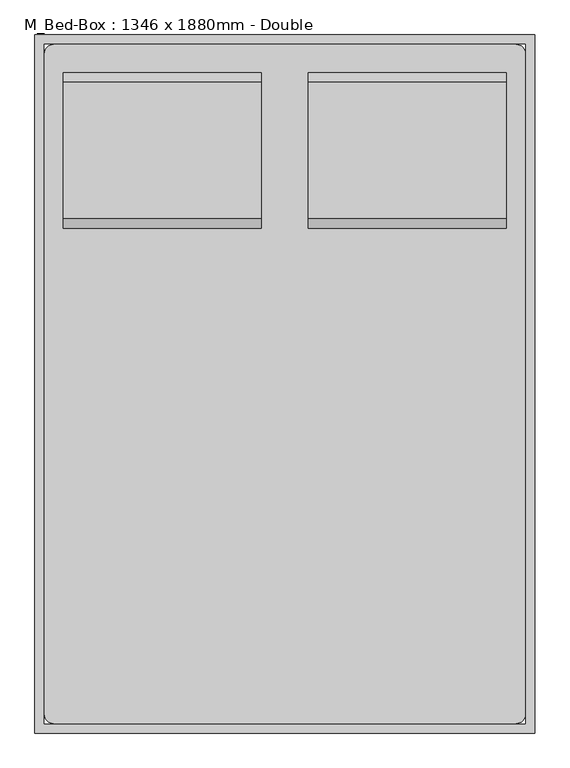
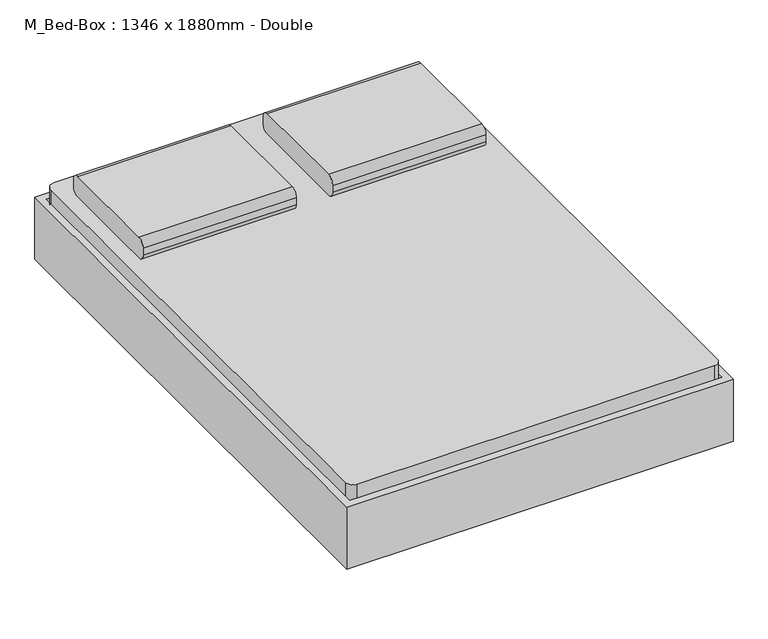
"""IFC4 building model written with IfcOpenShell, lengths in millimetres: furniture geometry, M_Bed-Box : 1346 x 1880mm - Double."""

from ifc_helpers import new_model, si_unit, point, frame, frame_2d, origin, place, context, project, spatial, polyline, circle_curve, trimmed, segment, composite_curve, outline, extrude, source, transform, mapped, element, save
from ifc_brep_helpers import plane_surface, cylinder_surface, revolved_surface, advanced_brep


def m_bed_box_1346_x_1880mm_double_52b0093e(model_context):
    return source(origin(), model_context, "Body", "SolidModel", [
        advanced_brep(
        [(-308.447541, -869.6295082, 196.85), (-308.447541, -869.6295082, 177.8), (-308.447541, -945.8295082, 177.8), (-308.447541, -945.8295082, 196.85), (-245.5113525, -869.6295082, 196.85), (-257.647541, -869.6295082, 177.8), (-257.647541, -945.8295082, 177.8), (-245.5113525, -945.8295082, 196.85), (-164.3115092, -869.6295082, 22.716374), (-181.5766725, -869.6295082, 14.6654962), (-181.5766725, -945.8295082, 14.6654962), (-164.3115092, -945.8295082, 22.716374), (-158.5564547, -869.6295082, 0.0), (-158.5564547, -869.6295082, 19.05), (-158.5564547, -945.8295082, 0.0), (-158.5564547, -945.8295082, 19.05), (-79.9439489, -869.6295082, 19.05), (-79.9439489, -869.6295082, 0.0), (-79.9439489, -945.8295082, 0.0), (-79.9439489, -945.8295082, 19.05), (-67.2439489, -869.6295082, 3.4029547), (-76.7689489, -869.6295082, 19.9007387), (-67.2439489, -945.8295082, 3.4029547), (-76.7689489, -945.8295082, 19.9007387), (-12.2513357, -869.6295082, 57.15), (-7.1469036, -869.6295082, 38.1), (-7.1469036, -945.8295082, 38.1), (-12.2513357, -945.8295082, 57.15), (690.5562537, -869.6295082, 57.15), (685.4518216, -869.6295082, 38.1), (685.4518216, -945.8295082, 38.1), (690.5562537, -945.8295082, 57.15), (755.0738669, -869.6295082, 19.9007387), (745.5488669, -869.6295082, 3.4029547), (745.5488669, -945.8295082, 3.4029547), (755.0738669, -945.8295082, 19.9007387), (758.2488669, -869.6295082, 0.0), (758.2488669, -869.6295082, 19.05), (758.2488669, -945.8295082, 0.0), (758.2488669, -945.8295082, 19.05), (836.8613728, -869.6295082, 19.05), (836.8613728, -869.6295082, 0.0), (836.8613728, -945.8295082, 0.0), (836.8613728, -945.8295082, 19.05), (859.8815906, -869.6295082, 14.6654962), (842.6164272, -869.6295082, 22.716374), (859.8815906, -945.8295082, 14.6654962), (842.6164272, -945.8295082, 22.716374), (923.8162705, -869.6295082, 196.85), (935.952459, -869.6295082, 177.8), (935.952459, -945.8295082, 177.8), (923.8162705, -945.8295082, 196.85), (986.752459, -869.6295082, 196.85), (986.752459, -945.8295082, 196.85), (986.752459, -945.8295082, 177.8), (986.752459, -869.6295082, 177.8)],
        [
            (0, 1),
            (1, 2),
            (2, 3),
            (3, 0),
            (0, 4),
            (4, 5),
            (5, 1),
            (5, 6),
            (6, 2),
            (6, 7),
            (7, 3),
            (7, 4),
            (4, 8),
            (8, 9),
            (9, 5),
            (9, 10),
            (10, 6),
            (10, 11),
            (11, 7),
            (11, 8),
            (12, 9, circle_curve(frame((-158.5564547, -869.6295082, 25.4), z_axis=(0.0, 1.0, 0.0), x_axis=(-0.9063077870366625, 0.0, -0.4226182617406725)), 25.4)),
            (8, 13, circle_curve(frame((-158.5564547, -869.6295082, 25.4), z_axis=(0.0, -1.0, 0.0), x_axis=(-0.9063077870366625, 0.0, -0.4226182617406725)), 6.35)),
            (13, 12),
            (14, 10, circle_curve(frame((-158.5564547, -945.8295082, 25.4), z_axis=(0.0, 1.0, 0.0), x_axis=(-0.9063077870366625, 0.0, -0.4226182617406725)), 25.4)),
            (12, 14),
            (15, 11, circle_curve(frame((-158.5564547, -945.8295082, 25.4), z_axis=(0.0, 1.0, 0.0), x_axis=(-0.9063077870366625, 0.0, -0.4226182617406725)), 6.35)),
            (14, 15),
            (15, 13),
            (13, 16),
            (16, 17),
            (17, 12),
            (17, 18),
            (18, 14),
            (18, 19),
            (19, 15),
            (19, 16),
            (20, 17, circle_curve(frame((-79.9439489, -869.6295082, 25.4), z_axis=(0.0, 1.0, 0.0), x_axis=(0.0, 0.0, -1.0)), 25.4)),
            (16, 21, circle_curve(frame((-79.9439489, -869.6295082, 25.4), z_axis=(0.0, -1.0, 0.0), x_axis=(0.0, 0.0, -1.0)), 6.35)),
            (21, 20),
            (22, 18, circle_curve(frame((-79.9439489, -945.8295082, 25.4), z_axis=(0.0, 1.0, 0.0), x_axis=(0.0, 0.0, -1.0)), 25.4)),
            (20, 22),
            (23, 19, circle_curve(frame((-79.9439489, -945.8295082, 25.4), z_axis=(0.0, 1.0, 0.0), x_axis=(0.0, 0.0, -1.0)), 6.35)),
            (22, 23),
            (23, 21),
            (21, 24),
            (24, 25),
            (25, 20),
            (25, 26),
            (26, 22),
            (26, 27),
            (27, 23),
            (27, 24),
            (24, 28),
            (28, 29),
            (29, 25),
            (29, 30),
            (30, 26),
            (30, 31),
            (31, 27),
            (31, 28),
            (28, 32),
            (32, 33),
            (33, 29),
            (33, 34),
            (34, 30),
            (34, 35),
            (35, 31),
            (35, 32),
            (36, 33, circle_curve(frame((758.2488669, -869.6295082, 25.4), z_axis=(0.0, 1.0, 0.0), x_axis=(-0.5000000000000528, 0.0, -0.8660254037844081)), 25.4)),
            (32, 37, circle_curve(frame((758.2488669, -869.6295082, 25.4), z_axis=(0.0, -1.0, 0.0), x_axis=(-0.5000000000000528, 0.0, -0.8660254037844081)), 6.35)),
            (37, 36),
            (38, 34, circle_curve(frame((758.2488669, -945.8295082, 25.4), z_axis=(0.0, 1.0, 0.0), x_axis=(-0.5000000000000528, 0.0, -0.8660254037844081)), 25.4)),
            (36, 38),
            (39, 35, circle_curve(frame((758.2488669, -945.8295082, 25.4), z_axis=(0.0, 1.0, 0.0), x_axis=(-0.5000000000000528, 0.0, -0.8660254037844081)), 6.35)),
            (38, 39),
            (39, 37),
            (37, 40),
            (40, 41),
            (41, 36),
            (41, 42),
            (42, 38),
            (42, 43),
            (43, 39),
            (43, 40),
            (44, 41, circle_curve(frame((836.8613728, -869.6295082, 25.4), z_axis=(0.0, 1.0, 0.0), x_axis=(0.0, 0.0, -1.0)), 25.4)),
            (40, 45, circle_curve(frame((836.8613728, -869.6295082, 25.4), z_axis=(0.0, -1.0, 0.0), x_axis=(0.0, 0.0, -1.0)), 6.35)),
            (45, 44),
            (46, 42, circle_curve(frame((836.8613728, -945.8295082, 25.4), z_axis=(0.0, 1.0, 0.0), x_axis=(0.0, 0.0, -1.0)), 25.4)),
            (44, 46),
            (47, 43, circle_curve(frame((836.8613728, -945.8295082, 25.4), z_axis=(0.0, 1.0, 0.0), x_axis=(0.0, 0.0, -1.0)), 6.35)),
            (46, 47),
            (47, 45),
            (45, 48),
            (48, 49),
            (49, 44),
            (49, 50),
            (50, 46),
            (50, 51),
            (51, 47),
            (51, 48),
            (52, 53),
            (53, 54),
            (54, 55),
            (55, 52),
            (48, 52),
            (55, 49),
            (54, 50),
            (53, 51),
        ],
        [
            plane_surface(frame((-308.447541, -1174.4295082, -127.5947323), z_axis=(-1.0, 0.0, 0.0), x_axis=(0.0, 1.0, 0.0))),
            plane_surface(frame((-308.447541, -869.6295082, 196.85), z_axis=(0.0, 1.0, 0.0), x_axis=(1.0, 0.0, 0.0))),
            plane_surface(frame((-308.447541, -869.6295082, 177.8), z_axis=(0.0, 0.0, -1.0), x_axis=(1.0, 0.0, 0.0))),
            plane_surface(frame((-308.447541, -945.8295082, 177.8), z_axis=(0.0, -1.0, 0.0), x_axis=(1.0, 0.0, 0.0))),
            plane_surface(frame((-308.447541, -945.8295082, 196.85), z_axis=(0.0, 0.0, 1.0), x_axis=(1.0, 0.0, 0.0))),
            plane_surface(frame((-245.5113525, -869.6295082, 196.85), z_axis=(0.0, 1.0, 0.0), x_axis=(0.4226182617406714, 0.0, -0.906307787036663))),
            plane_surface(frame((-257.647541, -869.6295082, 177.8), z_axis=(-0.9063077870366631, 0.0, -0.42261826174067146), x_axis=(0.42261826174067146, 0.0, -0.9063077870366631))),
            plane_surface(frame((-257.647541, -945.8295082, 177.8), z_axis=(0.0, -1.0000000000000002, 0.0), x_axis=(0.4226182617406716, 0.0, -0.906307787036663))),
            plane_surface(frame((-245.5113525, -945.8295082, 196.85), z_axis=(0.906307787036663, 0.0, 0.4226182617406716), x_axis=(0.4226182617406716, 0.0, -0.906307787036663))),
            plane_surface(frame((-158.5564547, -869.6295082, 25.4), z_axis=(0.0, 1.0, 0.0), x_axis=(-0.9063077870366625, 0.0, -0.4226182617406725))),
            cylinder_surface(frame((-158.5564547, -1174.4295082, 25.4), z_axis=(0.0, -1.0, 0.0), x_axis=(-0.9063077870366625, 0.0, -0.4226182617406725)), 25.4),
            plane_surface(frame((-158.5564547, -945.8295082, 25.4), z_axis=(0.0, -1.0, 0.0), x_axis=(-0.9063077870366625, 0.0, -0.4226182617406725))),
            revolved_surface(polyline([(-164.31150914768278, -945.8295082, 22.71637403794673), (-164.31150914768278, -869.6295082, 22.71637403794673)]), (-158.5564547, -1174.4295082, 25.4), (0.0, -1.0, 0.0)),
            plane_surface(frame((-158.5564547, -869.6295082, 19.05), z_axis=(0.0, 1.0, 0.0), x_axis=(1.0, 0.0, 0.0))),
            plane_surface(frame((-158.5564547, -869.6295082, 0.0), z_axis=(0.0, 0.0, -1.0), x_axis=(1.0, 0.0, 0.0))),
            plane_surface(frame((-158.5564547, -945.8295082, 0.0), z_axis=(0.0, -1.0, 0.0), x_axis=(1.0, 0.0, 0.0))),
            plane_surface(frame((-158.5564547, -945.8295082, 19.05), z_axis=(0.0, 0.0, 1.0), x_axis=(1.0, 0.0, 0.0))),
            plane_surface(frame((-79.9439489, -869.6295082, 25.4), z_axis=(0.0, 1.0, 0.0), x_axis=(0.0, 0.0, -1.0))),
            cylinder_surface(frame((-79.9439489, -1174.4295082, 25.4), z_axis=(0.0, -1.0, 0.0), x_axis=(0.0, 0.0, -1.0)), 25.4),
            plane_surface(frame((-79.9439489, -945.8295082, 25.4), z_axis=(0.0, -1.0, 0.0), x_axis=(0.0, 0.0, -1.0))),
            revolved_surface(polyline([(-79.9439489, -945.8295082, 19.049999999999997), (-79.9439489, -869.6295082, 19.049999999999997)]), (-79.9439489, -1174.4295082, 25.4), (0.0, -1.0, 0.0)),
            plane_surface(frame((-76.7689489, -869.6295082, 19.9007387), z_axis=(0.0, 1.0000000000000002, 0.0), x_axis=(0.8660254037844788, 0.0, 0.49999999999993067))),
            plane_surface(frame((-67.2439489, -869.6295082, 3.4029547), z_axis=(0.49999999999993067, 0.0, -0.8660254037844787), x_axis=(0.8660254037844787, 0.0, 0.49999999999993067))),
            plane_surface(frame((-67.2439489, -945.8295082, 3.4029547), z_axis=(0.0, -1.0, 0.0), x_axis=(0.8660254037844782, 0.0, 0.4999999999999315))),
            plane_surface(frame((-76.7689489, -945.8295082, 19.9007387), z_axis=(-0.49999999999993044, 0.0, 0.8660254037844789), x_axis=(0.8660254037844789, 0.0, 0.49999999999993044))),
            plane_surface(frame((-12.2513357, -869.6295082, 57.15), z_axis=(0.0, 1.0, 0.0), x_axis=(1.0, 0.0, 0.0))),
            plane_surface(frame((-7.1469036, -869.6295082, 38.1), z_axis=(0.0, 0.0, -1.0), x_axis=(1.0, 0.0, 0.0))),
            plane_surface(frame((-7.1469036, -945.8295082, 38.1), z_axis=(0.0, -1.0, 0.0), x_axis=(1.0, 0.0, 0.0))),
            plane_surface(frame((-12.2513357, -945.8295082, 57.15), z_axis=(0.0, 0.0, 1.0), x_axis=(1.0, 0.0, 0.0))),
            plane_surface(frame((690.5562537, -869.6295082, 57.15), z_axis=(0.0, 1.0, 0.0), x_axis=(0.8660254037844087, 0.0, -0.5000000000000518))),
            plane_surface(frame((685.4518216, -869.6295082, 38.1), z_axis=(-0.5000000000000513, 0.0, -0.8660254037844092), x_axis=(0.8660254037844092, 0.0, -0.5000000000000513))),
            plane_surface(frame((685.4518216, -945.8295082, 38.1), z_axis=(0.0, -1.0, 0.0), x_axis=(0.8660254037844081, 0.0, -0.5000000000000531))),
            plane_surface(frame((690.5562537, -945.8295082, 57.15), z_axis=(0.5000000000000521, 0.0, 0.8660254037844086), x_axis=(0.8660254037844086, 0.0, -0.5000000000000521))),
            plane_surface(frame((758.2488669, -869.6295082, 25.4), z_axis=(0.0, 1.0000000000000002, 0.0), x_axis=(-0.500000000000053, 0.0, -0.8660254037844082))),
            cylinder_surface(frame((758.2488669, -1174.4295082, 25.4), z_axis=(0.0, -1.0, 0.0), x_axis=(-0.5000000000000528, 0.0, -0.8660254037844081)), 25.4),
            plane_surface(frame((758.2488669, -945.8295082, 25.4), z_axis=(0.0, -1.0000000000000002, 0.0), x_axis=(-0.500000000000053, 0.0, -0.8660254037844082))),
            revolved_surface(polyline([(755.0738668999998, -945.8295082, 19.900738685969007), (755.0738668999998, -869.6295082, 19.900738685969007)]), (758.2488669, -1174.4295082, 25.4), (0.0, -1.0, 0.0)),
            plane_surface(frame((758.2488669, -869.6295082, 19.05), z_axis=(0.0, 1.0, 0.0), x_axis=(1.0, 0.0, 0.0))),
            plane_surface(frame((758.2488669, -869.6295082, 0.0), z_axis=(0.0, 0.0, -1.0), x_axis=(1.0, 0.0, 0.0))),
            plane_surface(frame((758.2488669, -945.8295082, 0.0), z_axis=(0.0, -1.0, 0.0), x_axis=(1.0, 0.0, 0.0))),
            plane_surface(frame((758.2488669, -945.8295082, 19.05), z_axis=(0.0, 0.0, 1.0), x_axis=(1.0, 0.0, 0.0))),
            plane_surface(frame((836.8613728, -869.6295082, 25.4), z_axis=(0.0, 1.0, 0.0), x_axis=(0.0, 0.0, -1.0))),
            cylinder_surface(frame((836.8613728, -1174.4295082, 25.4), z_axis=(0.0, -1.0, 0.0), x_axis=(0.0, 0.0, -1.0)), 25.4),
            plane_surface(frame((836.8613728, -945.8295082, 25.4), z_axis=(0.0, -1.0, 0.0), x_axis=(0.0, 0.0, -1.0))),
            revolved_surface(polyline([(836.8613728, -945.8295082, 19.049999999999997), (836.8613728, -869.6295082, 19.049999999999997)]), (836.8613728, -1174.4295082, 25.4), (0.0, -1.0, 0.0)),
            plane_surface(frame((842.6164272, -869.6295082, 22.716374), z_axis=(0.0, 1.0, 0.0), x_axis=(0.4226182617405387, 0.0, 0.906307787036725))),
            plane_surface(frame((859.8815906, -869.6295082, 14.6654962), z_axis=(0.906307787036725, 0.0, -0.4226182617405386), x_axis=(0.4226182617405386, 0.0, 0.906307787036725))),
            plane_surface(frame((859.8815906, -945.8295082, 14.6654962), z_axis=(0.0, -1.0, 0.0), x_axis=(0.4226182617405387, 0.0, 0.906307787036725))),
            plane_surface(frame((842.6164272, -945.8295082, 22.716374), z_axis=(-0.9063077870367251, 0.0, 0.4226182617405384), x_axis=(0.4226182617405384, 0.0, 0.9063077870367251))),
            plane_surface(frame((986.752459, -1174.4295082, -127.5947323), z_axis=(1.0, 0.0, 0.0), x_axis=(0.0, 1.0, 0.0))),
            plane_surface(frame((923.8162705, -869.6295082, 196.85), z_axis=(0.0, 1.0, 0.0), x_axis=(1.0, 0.0, 0.0))),
            plane_surface(frame((935.952459, -869.6295082, 177.8), z_axis=(0.0, 0.0, -1.0), x_axis=(1.0, 0.0, 0.0))),
            plane_surface(frame((935.952459, -945.8295082, 177.8), z_axis=(0.0, -1.0, 0.0), x_axis=(1.0, 0.0, 0.0))),
            plane_surface(frame((923.8162705, -945.8295082, 196.85), z_axis=(0.0, 0.0, 1.0), x_axis=(1.0, 0.0, 0.0))),
        ],
        [
            (0, [[1, 2, 3, 4]]),
            (1, [[-1, 5, 6, 7]]),
            (2, [[-2, -7, 8, 9]]),
            (3, [[-3, -9, 10, 11]]),
            (4, [[-4, -11, 12, -5]]),
            (5, [[-6, 13, 14, 15]]),
            (6, [[-8, -15, 16, 17]]),
            (7, [[-10, -17, 18, 19]]),
            (8, [[-12, -19, 20, -13]]),
            (9, [[21, -14, 22, 23]]),
            (10, [[24, -16, -21, 25]]),
            (11, [[26, -18, -24, 27]]),
            (12, [[-22, -20, -26, 28]]),
            (13, [[-23, 29, 30, 31]]),
            (14, [[-25, -31, 32, 33]]),
            (15, [[-27, -33, 34, 35]]),
            (16, [[-28, -35, 36, -29]]),
            (17, [[37, -30, 38, 39]]),
            (18, [[40, -32, -37, 41]]),
            (19, [[42, -34, -40, 43]]),
            (20, [[-38, -36, -42, 44]]),
            (21, [[-39, 45, 46, 47]]),
            (22, [[-41, -47, 48, 49]]),
            (23, [[-43, -49, 50, 51]]),
            (24, [[-44, -51, 52, -45]]),
            (25, [[-46, 53, 54, 55]]),
            (26, [[-48, -55, 56, 57]]),
            (27, [[-50, -57, 58, 59]]),
            (28, [[-52, -59, 60, -53]]),
            (29, [[-54, 61, 62, 63]]),
            (30, [[-56, -63, 64, 65]]),
            (31, [[-58, -65, 66, 67]]),
            (32, [[-60, -67, 68, -61]]),
            (33, [[69, -62, 70, 71]]),
            (34, [[72, -64, -69, 73]]),
            (35, [[74, -66, -72, 75]]),
            (36, [[-70, -68, -74, 76]]),
            (37, [[-71, 77, 78, 79]]),
            (38, [[-73, -79, 80, 81]]),
            (39, [[-75, -81, 82, 83]]),
            (40, [[-76, -83, 84, -77]]),
            (41, [[85, -78, 86, 87]]),
            (42, [[88, -80, -85, 89]]),
            (43, [[90, -82, -88, 91]]),
            (44, [[-86, -84, -90, 92]]),
            (45, [[-87, 93, 94, 95]]),
            (46, [[-89, -95, 96, 97]]),
            (47, [[-91, -97, 98, 99]]),
            (48, [[-92, -99, 100, -93]]),
            (49, [[101, 102, 103, 104]]),
            (50, [[-94, 105, -104, 106]]),
            (51, [[-96, -106, -103, 107]]),
            (52, [[-98, -107, -102, 108]]),
            (53, [[-100, -108, -101, -105]]),
        ],
    ),
        extrude(outline(composite_curve([segment(polyline([(-283.047541, 680.1704918), (961.352459, 680.1704918)]), True, "CONTINUOUS"), segment(trimmed(circle_curve(frame_2d((961.352459, 654.7704918)), 25.4), [point((961.352459, 680.1704918))], [point((986.752459, 654.7704918))], False, "CARTESIAN"), True, "CONTINUOUS"), segment(polyline([(986.752459, 654.7704918), (986.752459, -1123.6295082)]), True, "CONTINUOUS"), segment(trimmed(circle_curve(frame_2d((961.352459, -1123.6295082)), 25.4), [point((986.752459, -1123.6295082))], [point((961.352459, -1149.0295082))], False, "CARTESIAN"), True, "CONTINUOUS"), segment(polyline([(961.352459, -1149.0295082), (-283.047541, -1149.0295082)]), True, "CONTINUOUS"), segment(trimmed(circle_curve(frame_2d((-283.047541, -1123.6295082)), 25.4), [point((-283.047541, -1149.0295082))], [point((-308.447541, -1123.6295082))], False, "CARTESIAN"), True, "CONTINUOUS"), segment(polyline([(-308.447541, -1123.6295082), (-308.447541, 654.7704918)]), True, "CONTINUOUS"), segment(trimmed(circle_curve(frame_2d((-283.047541, 654.7704918)), 25.4), [point((-308.447541, 654.7704918))], [point((-283.047541, 680.1704918))], False, "CARTESIAN"), True, "CONTINUOUS")], self_intersect=False)), frame((0.0, 0.0, 203.2), z_axis=(0.0, 0.0, 1.0), x_axis=(1.0, 0.0, 0.0)), (0.0, 0.0, 1.0), 203.2),
        advanced_brep(
        [(-308.1231784, 451.5704918, 177.8), (-308.1231784, 375.3704918, 177.8), (-308.1231784, 375.3704918, 196.85), (-308.1231784, 451.5704918, 196.85), (-257.3231784, 451.5704918, 177.8), (-257.3231784, 375.3704918, 177.8), (-245.1869899, 375.3704918, 196.85), (-245.1869899, 451.5704918, 196.85), (-181.2523099, 451.5704918, 14.6654962), (-181.2523099, 375.3704918, 14.6654962), (-163.9871466, 375.3704918, 22.716374), (-163.9871466, 451.5704918, 22.716374), (-158.2320921, 375.3704918, 0.0), (-158.2320921, 451.5704918, 0.0), (-158.2320921, 375.3704918, 19.05), (-158.2320921, 451.5704918, 19.05), (-79.6195862, 451.5704918, 0.0), (-79.6195862, 375.3704918, 0.0), (-79.6195862, 375.3704918, 19.05), (-79.6195862, 451.5704918, 19.05), (-66.9195862, 375.3704918, 3.4029547), (-66.9195862, 451.5704918, 3.4029547), (-76.4445862, 375.3704918, 19.9007387), (-76.4445862, 451.5704918, 19.9007387), (-6.822541, 451.5704918, 38.1), (-6.822541, 375.3704918, 38.1), (-11.9269731, 375.3704918, 57.15), (-11.9269731, 451.5704918, 57.15), (685.4518216, 451.5704918, 38.1), (685.4518216, 375.3704918, 38.1), (690.5562537, 375.3704918, 57.15), (690.5562537, 451.5704918, 57.15), (745.5488669, 451.5704918, 3.4029547), (745.5488669, 375.3704918, 3.4029547), (755.0738669, 375.3704918, 19.9007387), (755.0738669, 451.5704918, 19.9007387), (758.2488669, 375.3704918, 0.0), (758.2488669, 451.5704918, 0.0), (758.2488669, 375.3704918, 19.05), (758.2488669, 451.5704918, 19.05), (836.8613728, 451.5704918, 0.0), (836.8613728, 375.3704918, 0.0), (836.8613728, 375.3704918, 19.05), (836.8613728, 451.5704918, 19.05), (859.8815906, 375.3704918, 14.6654962), (859.8815906, 451.5704918, 14.6654962), (842.6164272, 375.3704918, 22.716374), (842.6164272, 451.5704918, 22.716374), (935.952459, 451.5704918, 177.8), (935.952459, 375.3704918, 177.8), (923.8162705, 375.3704918, 196.85), (923.8162705, 451.5704918, 196.85), (986.752459, 451.5704918, 177.8), (986.752459, 451.5704918, 196.85), (986.752459, 375.3704918, 196.85), (986.752459, 375.3704918, 177.8)],
        [
            (0, 1),
            (1, 2),
            (2, 3),
            (3, 0),
            (0, 4),
            (4, 5),
            (5, 1),
            (5, 6),
            (6, 2),
            (6, 7),
            (7, 3),
            (7, 4),
            (4, 8),
            (8, 9),
            (9, 5),
            (9, 10),
            (10, 6),
            (10, 11),
            (11, 7),
            (11, 8),
            (12, 9, circle_curve(frame((-158.2320921, 375.3704918, 25.4), z_axis=(0.0, 1.0, 0.0), x_axis=(-0.906307787036649, 0.0, -0.4226182617407015)), 25.4)),
            (8, 13, circle_curve(frame((-158.2320921, 451.5704918, 25.4), z_axis=(0.0, -1.0, 0.0), x_axis=(-0.906307787036649, 0.0, -0.4226182617407015)), 25.4)),
            (13, 12),
            (14, 10, circle_curve(frame((-158.2320921, 375.3704918, 25.4), z_axis=(0.0, 1.0, 0.0), x_axis=(-0.906307787036649, 0.0, -0.4226182617407015)), 6.35)),
            (12, 14),
            (15, 11, circle_curve(frame((-158.2320921, 451.5704918, 25.4), z_axis=(0.0, 1.0, 0.0), x_axis=(-0.906307787036649, 0.0, -0.4226182617407015)), 6.35)),
            (14, 15),
            (15, 13),
            (13, 16),
            (16, 17),
            (17, 12),
            (17, 18),
            (18, 14),
            (18, 19),
            (19, 15),
            (19, 16),
            (20, 17, circle_curve(frame((-79.6195862, 375.3704918, 25.4), z_axis=(0.0, 1.0, 0.0), x_axis=(0.0, 0.0, -1.0)), 25.4)),
            (16, 21, circle_curve(frame((-79.6195862, 451.5704918, 25.4), z_axis=(0.0, -1.0, 0.0), x_axis=(0.0, 0.0, -1.0)), 25.4)),
            (21, 20),
            (22, 18, circle_curve(frame((-79.6195862, 375.3704918, 25.4), z_axis=(0.0, 1.0, 0.0), x_axis=(0.0, 0.0, -1.0)), 6.35)),
            (20, 22),
            (23, 19, circle_curve(frame((-79.6195862, 451.5704918, 25.4), z_axis=(0.0, 1.0, 0.0), x_axis=(0.0, 0.0, -1.0)), 6.35)),
            (22, 23),
            (23, 21),
            (21, 24),
            (24, 25),
            (25, 20),
            (25, 26),
            (26, 22),
            (26, 27),
            (27, 23),
            (27, 24),
            (24, 28),
            (28, 29),
            (29, 25),
            (29, 30),
            (30, 26),
            (30, 31),
            (31, 27),
            (31, 28),
            (28, 32),
            (32, 33),
            (33, 29),
            (33, 34),
            (34, 30),
            (34, 35),
            (35, 31),
            (35, 32),
            (36, 33, circle_curve(frame((758.2488669, 375.3704918, 25.4), z_axis=(0.0, 1.0, 0.0), x_axis=(-0.5000000000000463, 0.0, -0.8660254037844118)), 25.4)),
            (32, 37, circle_curve(frame((758.2488669, 451.5704918, 25.4), z_axis=(0.0, -1.0, 0.0), x_axis=(-0.5000000000000463, 0.0, -0.8660254037844118)), 25.4)),
            (37, 36),
            (38, 34, circle_curve(frame((758.2488669, 375.3704918, 25.4), z_axis=(0.0, 1.0, 0.0), x_axis=(-0.5000000000000463, 0.0, -0.8660254037844118)), 6.35)),
            (36, 38),
            (39, 35, circle_curve(frame((758.2488669, 451.5704918, 25.4), z_axis=(0.0, 1.0, 0.0), x_axis=(-0.5000000000000463, 0.0, -0.8660254037844118)), 6.35)),
            (38, 39),
            (39, 37),
            (37, 40),
            (40, 41),
            (41, 36),
            (41, 42),
            (42, 38),
            (42, 43),
            (43, 39),
            (43, 40),
            (44, 41, circle_curve(frame((836.8613728, 375.3704918, 25.4), z_axis=(0.0, 1.0, 0.0), x_axis=(0.0, 0.0, -1.0)), 25.4)),
            (40, 45, circle_curve(frame((836.8613728, 451.5704918, 25.4), z_axis=(0.0, -1.0, 0.0), x_axis=(0.0, 0.0, -1.0)), 25.4)),
            (45, 44),
            (46, 42, circle_curve(frame((836.8613728, 375.3704918, 25.4), z_axis=(0.0, 1.0, 0.0), x_axis=(0.0, 0.0, -1.0)), 6.35)),
            (44, 46),
            (47, 43, circle_curve(frame((836.8613728, 451.5704918, 25.4), z_axis=(0.0, 1.0, 0.0), x_axis=(0.0, 0.0, -1.0)), 6.35)),
            (46, 47),
            (47, 45),
            (45, 48),
            (48, 49),
            (49, 44),
            (49, 50),
            (50, 46),
            (50, 51),
            (51, 47),
            (51, 48),
            (52, 53),
            (53, 54),
            (54, 55),
            (55, 52),
            (48, 52),
            (55, 49),
            (54, 50),
            (53, 51),
        ],
        [
            plane_surface(frame((-308.1231784, 705.5704918, -152.9490627), z_axis=(-1.0, 0.0, 0.0), x_axis=(0.0, 1.0, 0.0))),
            plane_surface(frame((-308.1231784, 451.5704918, 177.8), z_axis=(0.0, 0.0, -1.0), x_axis=(1.0, 0.0, 0.0))),
            plane_surface(frame((-308.1231784, 375.3704918, 177.8), z_axis=(0.0, -1.0, 0.0), x_axis=(1.0, 0.0, 0.0))),
            plane_surface(frame((-308.1231784, 375.3704918, 196.85), z_axis=(0.0, 0.0, 1.0), x_axis=(1.0, 0.0, 0.0))),
            plane_surface(frame((-308.1231784, 451.5704918, 196.85), z_axis=(0.0, 1.0, 0.0), x_axis=(1.0, 0.0, 0.0))),
            plane_surface(frame((-257.3231784, 451.5704918, 177.8), z_axis=(-0.9063077870366486, 0.0, -0.4226182617407026), x_axis=(0.4226182617407026, 0.0, -0.9063077870366486))),
            plane_surface(frame((-257.3231784, 375.3704918, 177.8), z_axis=(0.0, -1.0000000000000002, 0.0), x_axis=(0.4226182617407026, 0.0, -0.9063077870366486))),
            plane_surface(frame((-245.1869899, 375.3704918, 196.85), z_axis=(0.9063077870366487, 0.0, 0.4226182617407023), x_axis=(0.4226182617407023, 0.0, -0.9063077870366487))),
            plane_surface(frame((-245.1869899, 451.5704918, 196.85), z_axis=(0.0, 1.0, 0.0), x_axis=(0.4226182617407027, 0.0, -0.9063077870366485))),
            cylinder_surface(frame((-158.2320921, 705.5704918, 25.4), z_axis=(0.0, -1.0, 0.0), x_axis=(-0.906307787036649, 0.0, -0.4226182617407015)), 25.4),
            plane_surface(frame((-158.2320921, 375.3704918, 25.4), z_axis=(0.0, -1.0, 0.0), x_axis=(-0.906307787036649, 0.0, -0.4226182617407015))),
            revolved_surface(polyline([(-163.9871465476827, 375.3704918, 22.716374037946544), (-163.9871465476827, 451.5704918, 22.716374037946544)]), (-158.2320921, 705.5704918, 25.4), (0.0, -1.0, 0.0)),
            plane_surface(frame((-158.2320921, 451.5704918, 25.4), z_axis=(0.0, 1.0, 0.0), x_axis=(-0.906307787036649, 0.0, -0.4226182617407015))),
            plane_surface(frame((-158.2320921, 451.5704918, 0.0), z_axis=(0.0, 0.0, -1.0), x_axis=(1.0, 0.0, 0.0))),
            plane_surface(frame((-158.2320921, 375.3704918, 0.0), z_axis=(0.0, -1.0, 0.0), x_axis=(1.0, 0.0, 0.0))),
            plane_surface(frame((-158.2320921, 375.3704918, 19.05), z_axis=(0.0, 0.0, 1.0), x_axis=(1.0, 0.0, 0.0))),
            plane_surface(frame((-158.2320921, 451.5704918, 19.05), z_axis=(0.0, 1.0, 0.0), x_axis=(1.0, 0.0, 0.0))),
            cylinder_surface(frame((-79.6195862, 705.5704918, 25.4), z_axis=(0.0, -1.0, 0.0), x_axis=(0.0, 0.0, -1.0)), 25.4),
            plane_surface(frame((-79.6195862, 375.3704918, 25.4), z_axis=(0.0, -1.0, 0.0), x_axis=(0.0, 0.0, -1.0))),
            revolved_surface(polyline([(-79.6195862, 375.3704918, 19.049999999999997), (-79.6195862, 451.5704918, 19.049999999999997)]), (-79.6195862, 705.5704918, 25.4), (0.0, -1.0, 0.0)),
            plane_surface(frame((-79.6195862, 451.5704918, 25.4), z_axis=(0.0, 1.0, 0.0), x_axis=(0.0, 0.0, -1.0))),
            plane_surface(frame((-66.9195862, 451.5704918, 3.4029547), z_axis=(0.4999999999998744, 0.0, -0.8660254037845112), x_axis=(0.8660254037845112, 0.0, 0.4999999999998744))),
            plane_surface(frame((-66.9195862, 375.3704918, 3.4029547), z_axis=(0.0, -1.0000000000000002, 0.0), x_axis=(0.8660254037845112, 0.0, 0.4999999999998745))),
            plane_surface(frame((-76.4445862, 375.3704918, 19.9007387), z_axis=(-0.4999999999998741, 0.0, 0.8660254037845113), x_axis=(0.8660254037845113, 0.0, 0.4999999999998741))),
            plane_surface(frame((-76.4445862, 451.5704918, 19.9007387), z_axis=(0.0, 1.0, 0.0), x_axis=(0.866025403784511, 0.0, 0.49999999999987477))),
            plane_surface(frame((-6.822541, 451.5704918, 38.1), z_axis=(0.0, 0.0, -1.0), x_axis=(1.0, 0.0, 0.0))),
            plane_surface(frame((-6.822541, 375.3704918, 38.1), z_axis=(0.0, -1.0, 0.0), x_axis=(1.0, 0.0, 0.0))),
            plane_surface(frame((-11.9269731, 375.3704918, 57.15), z_axis=(0.0, 0.0, 1.0), x_axis=(1.0, 0.0, 0.0))),
            plane_surface(frame((-11.9269731, 451.5704918, 57.15), z_axis=(0.0, 1.0, 0.0), x_axis=(1.0, 0.0, 0.0))),
            plane_surface(frame((685.4518216, 451.5704918, 38.1), z_axis=(-0.5000000000000494, 0.0, -0.8660254037844102), x_axis=(0.8660254037844102, 0.0, -0.5000000000000494))),
            plane_surface(frame((685.4518216, 375.3704918, 38.1), z_axis=(0.0, -1.0, 0.0), x_axis=(0.8660254037844112, 0.0, -0.5000000000000476))),
            plane_surface(frame((690.5562537, 375.3704918, 57.15), z_axis=(0.5000000000000488, 0.0, 0.8660254037844105), x_axis=(0.8660254037844105, 0.0, -0.5000000000000488))),
            plane_surface(frame((690.5562537, 451.5704918, 57.15), z_axis=(0.0, 1.0, 0.0), x_axis=(0.8660254037844106, 0.0, -0.5000000000000485))),
            cylinder_surface(frame((758.2488669, 705.5704918, 25.4), z_axis=(0.0, -1.0, 0.0), x_axis=(-0.5000000000000463, 0.0, -0.8660254037844118)), 25.4),
            plane_surface(frame((758.2488669, 375.3704918, 25.4), z_axis=(0.0, -1.0000000000000002, 0.0), x_axis=(-0.5000000000000464, 0.0, -0.866025403784412))),
            revolved_surface(polyline([(755.0738668999998, 375.3704918, 19.90073868596898), (755.0738668999998, 451.5704918, 19.90073868596898)]), (758.2488669, 705.5704918, 25.4), (0.0, -1.0, 0.0)),
            plane_surface(frame((758.2488669, 451.5704918, 25.4), z_axis=(0.0, 1.0000000000000002, 0.0), x_axis=(-0.5000000000000464, 0.0, -0.866025403784412))),
            plane_surface(frame((758.2488669, 451.5704918, 0.0), z_axis=(0.0, 0.0, -1.0), x_axis=(1.0, 0.0, 0.0))),
            plane_surface(frame((758.2488669, 375.3704918, 0.0), z_axis=(0.0, -1.0, 0.0), x_axis=(1.0, 0.0, 0.0))),
            plane_surface(frame((758.2488669, 375.3704918, 19.05), z_axis=(0.0, 0.0, 1.0), x_axis=(1.0, 0.0, 0.0))),
            plane_surface(frame((758.2488669, 451.5704918, 19.05), z_axis=(0.0, 1.0, 0.0), x_axis=(1.0, 0.0, 0.0))),
            cylinder_surface(frame((836.8613728, 705.5704918, 25.4), z_axis=(0.0, -1.0, 0.0), x_axis=(0.0, 0.0, -1.0)), 25.4),
            plane_surface(frame((836.8613728, 375.3704918, 25.4), z_axis=(0.0, -1.0, 0.0), x_axis=(0.0, 0.0, -1.0))),
            revolved_surface(polyline([(836.8613728, 375.3704918, 19.049999999999997), (836.8613728, 451.5704918, 19.049999999999997)]), (836.8613728, 705.5704918, 25.4), (0.0, -1.0, 0.0)),
            plane_surface(frame((836.8613728, 451.5704918, 25.4), z_axis=(0.0, 1.0, 0.0), x_axis=(0.0, 0.0, -1.0))),
            plane_surface(frame((859.8815906, 451.5704918, 14.6654962), z_axis=(0.90630778703668, 0.0, -0.422618261740635), x_axis=(0.422618261740635, 0.0, 0.90630778703668))),
            plane_surface(frame((859.8815906, 375.3704918, 14.6654962), z_axis=(0.0, -1.0000000000000002, 0.0), x_axis=(0.4226182617406349, 0.0, 0.9063077870366801))),
            plane_surface(frame((842.6164272, 375.3704918, 22.716374), z_axis=(-0.9063077870366805, 0.0, 0.4226182617406341), x_axis=(0.4226182617406341, 0.0, 0.9063077870366805))),
            plane_surface(frame((842.6164272, 451.5704918, 22.716374), z_axis=(0.0, 1.0, 0.0), x_axis=(0.42261826174063455, 0.0, 0.9063077870366802))),
            plane_surface(frame((986.752459, 705.5704918, -152.9490627), z_axis=(1.0, 0.0, 0.0), x_axis=(0.0, 1.0, 0.0))),
            plane_surface(frame((935.952459, 451.5704918, 177.8), z_axis=(0.0, 0.0, -1.0), x_axis=(1.0, 0.0, 0.0))),
            plane_surface(frame((935.952459, 375.3704918, 177.8), z_axis=(0.0, -1.0, 0.0), x_axis=(1.0, 0.0, 0.0))),
            plane_surface(frame((923.8162705, 375.3704918, 196.85), z_axis=(0.0, 0.0, 1.0), x_axis=(1.0, 0.0, 0.0))),
            plane_surface(frame((923.8162705, 451.5704918, 196.85), z_axis=(0.0, 1.0, 0.0), x_axis=(1.0, 0.0, 0.0))),
        ],
        [
            (0, [[1, 2, 3, 4]]),
            (1, [[-1, 5, 6, 7]]),
            (2, [[-2, -7, 8, 9]]),
            (3, [[-3, -9, 10, 11]]),
            (4, [[-4, -11, 12, -5]]),
            (5, [[-6, 13, 14, 15]]),
            (6, [[-8, -15, 16, 17]]),
            (7, [[-10, -17, 18, 19]]),
            (8, [[-12, -19, 20, -13]]),
            (9, [[21, -14, 22, 23]]),
            (10, [[24, -16, -21, 25]]),
            (11, [[26, -18, -24, 27]]),
            (12, [[-22, -20, -26, 28]]),
            (13, [[-23, 29, 30, 31]]),
            (14, [[-25, -31, 32, 33]]),
            (15, [[-27, -33, 34, 35]]),
            (16, [[-28, -35, 36, -29]]),
            (17, [[37, -30, 38, 39]]),
            (18, [[40, -32, -37, 41]]),
            (19, [[42, -34, -40, 43]]),
            (20, [[-38, -36, -42, 44]]),
            (21, [[-39, 45, 46, 47]]),
            (22, [[-41, -47, 48, 49]]),
            (23, [[-43, -49, 50, 51]]),
            (24, [[-44, -51, 52, -45]]),
            (25, [[-46, 53, 54, 55]]),
            (26, [[-48, -55, 56, 57]]),
            (27, [[-50, -57, 58, 59]]),
            (28, [[-52, -59, 60, -53]]),
            (29, [[-54, 61, 62, 63]]),
            (30, [[-56, -63, 64, 65]]),
            (31, [[-58, -65, 66, 67]]),
            (32, [[-60, -67, 68, -61]]),
            (33, [[69, -62, 70, 71]]),
            (34, [[72, -64, -69, 73]]),
            (35, [[74, -66, -72, 75]]),
            (36, [[-70, -68, -74, 76]]),
            (37, [[-71, 77, 78, 79]]),
            (38, [[-73, -79, 80, 81]]),
            (39, [[-75, -81, 82, 83]]),
            (40, [[-76, -83, 84, -77]]),
            (41, [[85, -78, 86, 87]]),
            (42, [[88, -80, -85, 89]]),
            (43, [[90, -82, -88, 91]]),
            (44, [[-86, -84, -90, 92]]),
            (45, [[-87, 93, 94, 95]]),
            (46, [[-89, -95, 96, 97]]),
            (47, [[-91, -97, 98, 99]]),
            (48, [[-92, -99, 100, -93]]),
            (49, [[101, 102, 103, 104]]),
            (50, [[-94, 105, -104, 106]]),
            (51, [[-96, -106, -103, 107]]),
            (52, [[-98, -107, -102, 108]]),
            (53, [[-100, -108, -101, -105]]),
        ],
    ),
        extrude(outline(composite_curve([segment(polyline([(578.5704918, 406.4), (210.2704918, 406.4)]), True, "CONTINUOUS"), segment(trimmed(circle_curve(frame_2d((210.2704918, 431.8)), 25.4), [point((210.2704918, 406.4))], [point((184.8704918, 431.8))], False, "CARTESIAN"), True, "CONTINUOUS"), segment(polyline([(184.8704918, 431.8), (184.8704918, 457.2)]), True, "CONTINUOUS"), segment(trimmed(circle_curve(frame_2d((210.2704918, 457.2)), 25.4), [point((184.8704918, 457.2))], [point((210.2704918, 482.6))], False, "CARTESIAN"), True, "CONTINUOUS"), segment(polyline([(210.2704918, 482.6), (578.5704918, 482.6)]), True, "CONTINUOUS"), segment(trimmed(circle_curve(frame_2d((578.5704918, 457.2)), 25.4), [point((578.5704918, 482.6))], [point((603.9704918, 457.2))], False, "CARTESIAN"), True, "CONTINUOUS"), segment(polyline([(603.9704918, 457.2), (603.9704918, 431.8)]), True, "CONTINUOUS"), segment(trimmed(circle_curve(frame_2d((578.5704918, 431.8)), 25.4), [point((603.9704918, 431.8))], [point((578.5704918, 406.4))], False, "CARTESIAN"), True, "CONTINUOUS")], self_intersect=False)), frame((-257.647541, 0.0, 0.0), z_axis=(1.0, 0.0, 0.0), x_axis=(0.0, 1.0, 0.0)), (0.0, 0.0, 1.0), 533.3),
        extrude(outline(composite_curve([segment(polyline([(578.5704918, 406.4), (210.2704918, 406.4)]), True, "CONTINUOUS"), segment(trimmed(circle_curve(frame_2d((210.2704918, 431.8)), 25.4), [point((210.2704918, 406.4))], [point((184.8704918, 431.8))], False, "CARTESIAN"), True, "CONTINUOUS"), segment(polyline([(184.8704918, 431.8), (184.8704918, 457.2)]), True, "CONTINUOUS"), segment(trimmed(circle_curve(frame_2d((210.2704918, 457.2)), 25.4), [point((184.8704918, 457.2))], [point((210.2704918, 482.6))], False, "CARTESIAN"), True, "CONTINUOUS"), segment(polyline([(210.2704918, 482.6), (578.5704918, 482.6)]), True, "CONTINUOUS"), segment(trimmed(circle_curve(frame_2d((578.5704918, 457.2)), 25.4), [point((578.5704918, 482.6))], [point((603.9704918, 457.2))], False, "CARTESIAN"), True, "CONTINUOUS"), segment(polyline([(603.9704918, 457.2), (603.9704918, 431.8)]), True, "CONTINUOUS"), segment(trimmed(circle_curve(frame_2d((578.5704918, 431.8)), 25.4), [point((603.9704918, 431.8))], [point((578.5704918, 406.4))], False, "CARTESIAN"), True, "CONTINUOUS")], self_intersect=False)), frame((402.652459, 0.0, 0.0), z_axis=(1.0, 0.0, 0.0), x_axis=(0.0, 1.0, 0.0)), (0.0, 0.0, 1.0), 533.3),
        extrude(outline(polyline([(1012.152459, 705.5704918), (1012.152459, -1174.4295082), (-333.847541, -1174.4295082), (-333.847541, 705.5704918), (1012.152459, 705.5704918)]), holes=[polyline([(986.752459, 680.1704918), (-308.447541, 680.1704918), (-308.447541, -1149.0295082), (986.752459, -1149.0295082), (986.752459, 680.1704918)])]), frame((0.0, 0.0, 127.0), z_axis=(0.0, 0.0, 1.0), x_axis=(1.0, 0.0, 0.0)), (0.0, 0.0, 1.0), 228.6),
    ])


if __name__ == "__main__":
    model = new_model("IFC4")
    model_context = context("Model", 3, world=origin())
    ifc_project = project(units=[si_unit("LENGTHUNIT", "METRE", prefix="MILLI")], contexts=[model_context])
    site = spatial("IfcSite", under=ifc_project)
    building = spatial("IfcBuilding", under=site)
    placement = place(None, origin())
    m_bed_box_1346_x_1880mm_double_shape = m_bed_box_1346_x_1880mm_double_52b0093e(model_context)
    element("IfcFurniture", 1, ObjectType="M_Bed-Box : 1346 x 1880mm - Double", at=placement, inside=building, context=model_context, shape_type="MappedRepresentation", body=[
        mapped(m_bed_box_1346_x_1880mm_double_shape, transform((0.0, 0.0, 0.0), x_axis=(1.0, 0.0, 0.0), y_axis=(0.0, 1.0, 0.0), z_axis=(0.0, 0.0, 1.0))),
    ])
    save(model, "model.ifc")

# Revit data of these elements
# Type "M_Bed-Box : 1346 x 1880mm - Double"
#   Length = 1880 mm
#   Width = 1346 mm
#   Frame Material = Birch
#   Mattress Material = Linen, White
#   Default Elevation = 0
# Element 1 (IfcFurniture, "M_Bed-Box : 1346 x 1880mm - Double")
#   Materials on its faces: "Birch", "Linen, White"
# Materials
#   "Birch": class "Wood", colour RGB 224 178 126, transparency 0, Description = "Betula Alleghaniensis", Cost = 0
#   "Linen, White": class "Textile", colour RGB 247 247 239, transparency 0, Description = "Linen, white", Cost = 0
